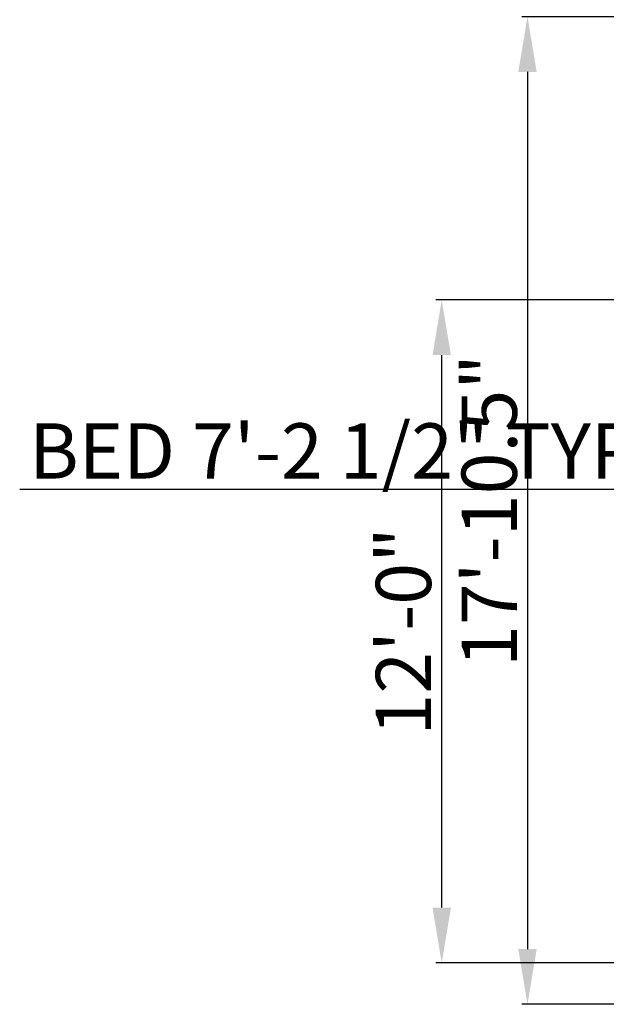
# Model space of a CAD drawing. Units: inches. Extents: x 2083 to 3317, y 1141 to 2115.
# Tile 1 of 256: x 2083 to 2210, y 1263 to 1477. Entities that reach past the tile are written whole.
import ezdxf

# ---------------------------------------------------------------- set-up
doc = ezdxf.new("R2010")
doc.units = ezdxf.units.IN
doc.layers.add('A-ANNO-DIMS', color=2, linetype='Continuous', lineweight=18)
doc.styles.get("Standard").update_dxf_attribs({"font": 'arial.ttf'})
doc.dimstyles.new('ISO-25', dxfattribs={"dimtxt": 12, "dimasz": 12, "dimexe": 1.25, "dimexo": 0.625, "dimtad": 1, "dimlunit": 3, "dimtxsty": 'Standard', "dimcen": 2.5, "dimadec": 0, "dimazin": 0, "dimtfac": 1, "dimtmove": 0, "dimatfit": 3, "dimfxl": 1, "dimarcsym": 0})

# ---------------------------------------------------------------- blocks, each defined once
blk = doc.blocks.new('*D13')
at = {"layer": 'A-ANNO-DIMS', "color": 0, "lineweight": -2, "transparency": 16777216}
for p, q in [((2226.33, 1477.76), (2191.98, 1477.76)), ((2193.23, 1465.76), (2193.23, 1275.26)), ((2226.33, 1263.26), (2191.98, 1263.26))]:
    blk.add_line(p, q, dxfattribs=at)
at = {"layer": 'A-ANNO-DIMS', "color": 0, "transparency": 16777216}
for points in [[(2191.23, 1465.76), (2195.23, 1465.76), (2193.23, 1477.76)], [(2191.23, 1275.26), (2195.23, 1275.26), (2193.23, 1263.26)]]:
    blk.add_solid(points, dxfattribs=at)
at = {"layer": 'Defpoints', "color": 0, "transparency": 16777216}
for p in [(2226.96, 1477.76), (2193.23, 1263.26), (2226.96, 1263.26)]:
    blk.add_point(p, dxfattribs=at)
at = {"layer": 'A-ANNO-DIMS', "color": 0, "transparency": 16777216, "insert": (2186.47, 1370.51), "char_height": 12, "attachment_point": 5, "rotation": 90}
blk.add_mtext('17\'-10.5"', dxfattribs=at)
blk = doc.blocks.new('*D22')
at = {"layer": 'A-ANNO-DIMS', "color": 0, "lineweight": -2, "transparency": 16777216}
for p, q in [((2235.96, 1362.74), (2235.96, 1376.31)), ((2322.26, 1362.74), (2322.26, 1376.31)), ((2235.96, 1375.06), (2083.01, 1375.06)), ((2310.26, 1375.06), (2247.96, 1375.06))]:
    blk.add_line(p, q, dxfattribs=at)
at = {"layer": 'A-ANNO-DIMS', "color": 0, "transparency": 16777216}
for points in [[(2247.96, 1377.06), (2247.96, 1373.06), (2235.96, 1375.06)], [(2310.26, 1377.06), (2310.26, 1373.06), (2322.26, 1375.06)]]:
    blk.add_solid(points, dxfattribs=at)
at = {"layer": 'Defpoints', "color": 0, "transparency": 16777216}
for p in [(2235.96, 1375.06), (2235.96, 1362.11), (2322.26, 1362.11)]:
    blk.add_point(p, dxfattribs=at)
at = {"layer": 'A-ANNO-DIMS', "color": 0, "transparency": 16777216, "insert": (2153.48, 1381.89), "char_height": 12, "attachment_point": 5}
blk.add_mtext('BED 7\'-2 1/2" TYP.', dxfattribs=at)
blk = doc.blocks.new('*D47')
at = {"layer": 'A-ANNO-DIMS', "color": 0, "lineweight": -2, "transparency": 16777216}
for p, q in [((2235.33, 1416.26), (2173.36, 1416.26)), ((2174.61, 1284.26), (2174.61, 1404.26)), ((2235.33, 1272.26), (2173.36, 1272.26))]:
    blk.add_line(p, q, dxfattribs=at)
at = {"layer": 'A-ANNO-DIMS', "color": 0, "transparency": 16777216}
for points in [[(2172.61, 1404.26), (2176.61, 1404.26), (2174.61, 1416.26)], [(2172.61, 1284.26), (2176.61, 1284.26), (2174.61, 1272.26)]]:
    blk.add_solid(points, dxfattribs=at)
at = {"layer": 'Defpoints', "color": 0, "transparency": 16777216}
for p in [(2174.61, 1416.26), (2235.96, 1416.26), (2235.96, 1272.26)]:
    blk.add_point(p, dxfattribs=at)
at = {"layer": 'A-ANNO-DIMS', "color": 0, "transparency": 16777216, "insert": (2167.86, 1344.26), "char_height": 12, "attachment_point": 5, "rotation": 90}
blk.add_mtext('12\'-0"', dxfattribs=at)

msp = doc.modelspace()

# ---------------------------------------------------------------- dimensions: what is measured, and where the dimension line sits
at = {"layer": 'A-ANNO-DIMS'}
for base, p1, p2, override, picture, middle in [((2193.226, 1263.261), (2226.96, 1477.761), (2226.96, 1263.261), {"dimclrd": 0, "dimclre": 0, "dimclrt": 0}, '*D13', (2186.474, 1370.511)), ((2174.61, 1416.261), (2235.96, 1272.261), (2235.96, 1416.261), {"dimdec": 1, "dimlfac": 1, "dimrnd": 0, "dimzin": 1, "dimdsep": 46, "dimlunit": 4, "dimfrac": 2}, '*D47', (2167.858, 1344.261))]:
    dim = msp.add_linear_dim(base=base, p1=p1, p2=p2, angle=90, dimstyle='ISO-25', override=override, dxfattribs=at)
    dim.commit()
    dim.dimension.update_dxf_attribs({"geometry": picture, "text_midpoint": middle})
dim = msp.add_linear_dim(base=(2235.96, 1375.059), p1=(2322.26, 1362.114), p2=(2235.96, 1362.114), angle=180, text='BED <> TYP.', dimstyle='ISO-25', override={"dimdec": 1, "dimlfac": 1, "dimrnd": 0, "dimzin": 1, "dimdsep": 46, "dimlunit": 4, "dimfrac": 2}, dxfattribs=at)
dim.commit()
dim.dimension.update_dxf_attribs({"geometry": '*D22', "text_midpoint": (2153.483, 1381.889)})

doc.saveas('drawing.dxf')
